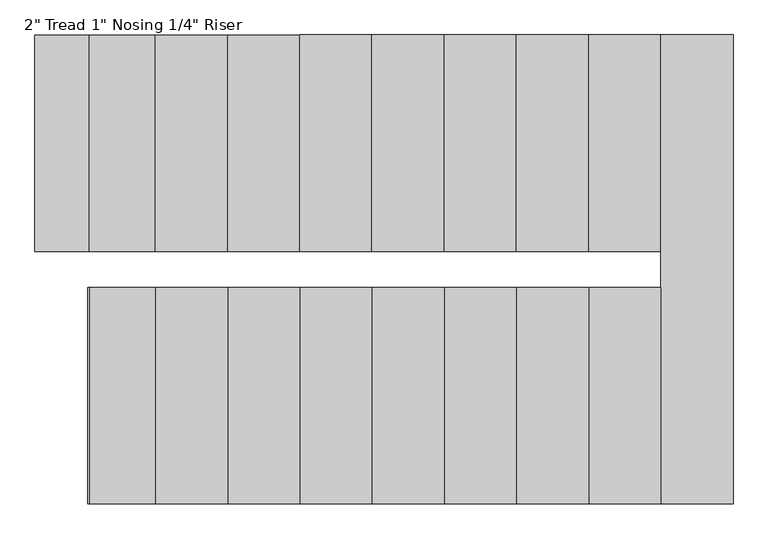
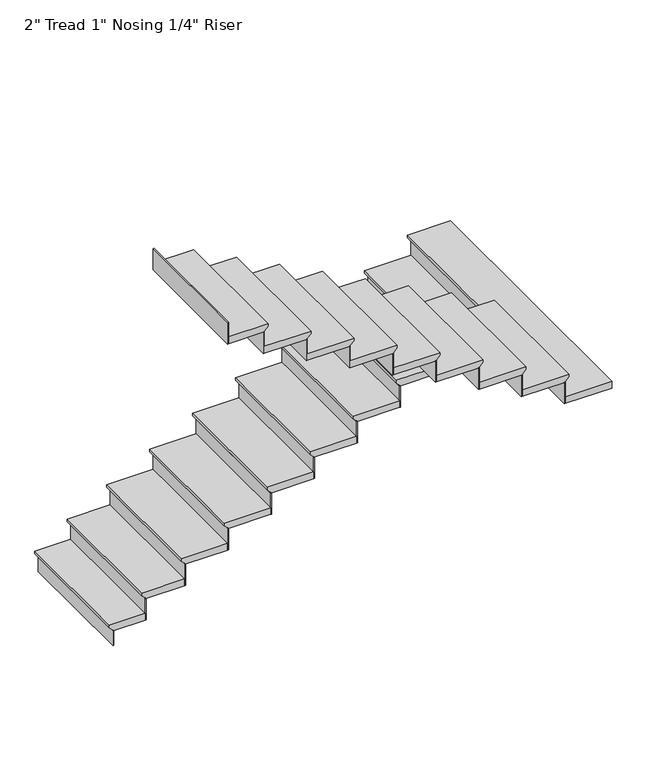
"""IFC4 building model written with IfcOpenShell, lengths in millimetres: stair flight geometry."""

from ifc_helpers import new_model, si_unit, origin, place, context, project, spatial, faceted_brep, source, transform, mapped, element, save


def stair_flight_a6cfe23b(model_context):
    return source(origin(), model_context, "Body", "Brep", [
        faceted_brep([(8572.5, 8280.4, 6237.3710526), (8572.5, 8280.4, 6256.4210526), (8572.5, 9194.8, 6256.4210526), (8572.5, 9194.8, 6237.3710526), (8597.9, 8280.4, 6211.9710526), (8597.9, 9194.8, 6211.9710526), (8826.5, 8280.4, 6256.4210526), (8826.5, 9194.8, 6256.4210526), (8597.9, 9194.8, 6205.6210526), (8826.5, 9194.8, 6205.6210526), (8826.5, 8280.4, 6205.6210526), (8597.9, 8280.4, 6205.6210526)], [[[0, 1, 2, 3]], [[4, 0, 3, 5]], [[2, 1, 6, 7]], [[8, 9, 10, 11]], [[2, 7, 9, 8, 5, 3]], [[8, 11, 4, 5]], [[6, 1, 0, 4, 11, 10]], [[7, 6, 10, 9]]]),
        faceted_brep([(8597.9, 8280.4, 6205.6210526), (8597.9, 8280.4, 6096.0), (8604.25, 8280.4, 6096.0), (8604.25, 8280.4, 6205.6210526), (8597.9, 9194.8, 6205.6210526), (8604.25, 9194.8, 6205.6210526), (8604.25, 9194.8, 6096.0), (8597.9, 9194.8, 6096.0)], [[[0, 1, 2, 3]], [[4, 5, 6, 7]], [[1, 0, 4, 7]], [[2, 1, 7, 6]], [[3, 2, 6, 5]], [[0, 3, 5, 4]]]),
        faceted_brep([(8826.5, 8280.4, 6366.0421053), (8826.5, 8280.4, 6205.6210526), (8832.85, 8280.4, 6205.6210526), (8832.85, 8280.4, 6366.0421053), (8826.5, 9194.8, 6366.0421053), (8832.85, 9194.8, 6366.0421053), (8832.85, 9194.8, 6205.6210526), (8826.5, 9194.8, 6205.6210526)], [[[0, 1, 2, 3]], [[4, 5, 6, 7]], [[1, 0, 4, 7]], [[2, 1, 7, 6]], [[3, 2, 6, 5]], [[0, 3, 5, 4]]]),
        faceted_brep([(8801.1, 9194.8, 6416.8421053), (8801.1, 8280.4, 6416.8421053), (9105.9, 8280.4, 6416.8421053), (9105.9, 9194.8, 6416.8421053), (8826.5, 9194.8, 6366.0421053), (9105.9, 9194.8, 6366.0421053), (9105.9, 8280.4, 6366.0421053), (8826.5, 8280.4, 6366.0421053), (8826.5, 9194.8, 6372.3921053), (8801.1, 9194.8, 6397.7921053), (8826.5, 8280.4, 6372.3921053), (8801.1, 8280.4, 6397.7921053)], [[[0, 1, 2, 3]], [[4, 5, 6, 7]], [[0, 3, 5, 4, 8, 9]], [[4, 7, 10, 8]], [[2, 1, 11, 10, 7, 6]], [[3, 2, 6, 5]], [[11, 1, 0, 9]], [[10, 11, 9, 8]]]),
        faceted_brep([(9105.9, 8280.4, 6526.4631579), (9105.9, 8280.4, 6366.0421053), (9112.25, 8280.4, 6366.0421053), (9112.25, 8280.4, 6526.4631579), (9105.9, 9194.8, 6526.4631579), (9112.25, 9194.8, 6526.4631579), (9112.25, 9194.8, 6366.0421053), (9105.9, 9194.8, 6366.0421053)], [[[0, 1, 2, 3]], [[4, 5, 6, 7]], [[1, 0, 4, 7]], [[2, 1, 7, 6]], [[3, 2, 6, 5]], [[0, 3, 5, 4]]]),
        faceted_brep([(9080.5, 9194.8, 6577.2631579), (9080.5, 8280.4, 6577.2631579), (9410.7, 8280.4, 6577.2631579), (9410.7, 9194.8, 6577.2631579), (9105.9, 9194.8, 6526.4631579), (9410.7, 9194.8, 6526.4631579), (9410.7, 8280.4, 6526.4631579), (9105.9, 8280.4, 6526.4631579), (9105.9, 9194.8, 6532.8131579), (9080.5, 9194.8, 6558.2131579), (9105.9, 8280.4, 6532.8131579), (9080.5, 8280.4, 6558.2131579)], [[[0, 1, 2, 3]], [[4, 5, 6, 7]], [[0, 3, 5, 4, 8, 9]], [[4, 7, 10, 8]], [[2, 1, 11, 10, 7, 6]], [[3, 2, 6, 5]], [[11, 1, 0, 9]], [[10, 11, 9, 8]]]),
        faceted_brep([(9410.7, 8280.4, 6686.8842105), (9410.7, 8280.4, 6526.4631579), (9417.05, 8280.4, 6526.4631579), (9417.05, 8280.4, 6686.8842105), (9410.7, 9194.8, 6686.8842105), (9417.05, 9194.8, 6686.8842105), (9417.05, 9194.8, 6526.4631579), (9410.7, 9194.8, 6526.4631579)], [[[0, 1, 2, 3]], [[4, 5, 6, 7]], [[1, 0, 4, 7]], [[2, 1, 7, 6]], [[3, 2, 6, 5]], [[0, 3, 5, 4]]]),
        faceted_brep([(9385.3, 9194.8, 6737.6842105), (9385.3, 8280.4, 6737.6842105), (9715.5, 8280.4, 6737.6842105), (9715.5, 9194.8, 6737.6842105), (9410.7, 9194.8, 6686.8842105), (9715.5, 9194.8, 6686.8842105), (9715.5, 8280.4, 6686.8842105), (9410.7, 8280.4, 6686.8842105), (9410.7, 9194.8, 6693.2342105), (9385.3, 9194.8, 6718.6342105), (9410.7, 8280.4, 6693.2342105), (9385.3, 8280.4, 6718.6342105)], [[[0, 1, 2, 3]], [[4, 5, 6, 7]], [[0, 3, 5, 4, 8, 9]], [[4, 7, 10, 8]], [[2, 1, 11, 10, 7, 6]], [[3, 2, 6, 5]], [[11, 1, 0, 9]], [[10, 11, 9, 8]]]),
        faceted_brep([(9715.5, 8280.4, 6847.3052632), (9715.5, 8280.4, 6686.8842105), (9721.85, 8280.4, 6686.8842105), (9721.85, 8280.4, 6847.3052632), (9715.5, 9194.8, 6847.3052632), (9721.85, 9194.8, 6847.3052632), (9721.85, 9194.8, 6686.8842105), (9715.5, 9194.8, 6686.8842105)], [[[0, 1, 2, 3]], [[4, 5, 6, 7]], [[1, 0, 4, 7]], [[2, 1, 7, 6]], [[3, 2, 6, 5]], [[0, 3, 5, 4]]]),
        faceted_brep([(9690.1, 9194.8, 6898.1052632), (9690.1, 8280.4, 6898.1052632), (10020.3, 8280.4, 6898.1052632), (10020.3, 9194.8, 6898.1052632), (9715.5, 9194.8, 6847.3052632), (10020.3, 9194.8, 6847.3052632), (10020.3, 8280.4, 6847.3052632), (9715.5, 8280.4, 6847.3052632), (9715.5, 9194.8, 6853.6552632), (9690.1, 9194.8, 6879.0552632), (9715.5, 8280.4, 6853.6552632), (9690.1, 8280.4, 6879.0552632)], [[[0, 1, 2, 3]], [[4, 5, 6, 7]], [[0, 3, 5, 4, 8, 9]], [[4, 7, 10, 8]], [[2, 1, 11, 10, 7, 6]], [[3, 2, 6, 5]], [[11, 1, 0, 9]], [[10, 11, 9, 8]]]),
        faceted_brep([(10020.3, 8280.4, 7007.7263158), (10020.3, 8280.4, 6847.3052632), (10026.65, 8280.4, 6847.3052632), (10026.65, 8280.4, 7007.7263158), (10020.3, 9194.8, 7007.7263158), (10026.65, 9194.8, 7007.7263158), (10026.65, 9194.8, 6847.3052632), (10020.3, 9194.8, 6847.3052632)], [[[0, 1, 2, 3]], [[4, 5, 6, 7]], [[1, 0, 4, 7]], [[2, 1, 7, 6]], [[3, 2, 6, 5]], [[0, 3, 5, 4]]]),
        faceted_brep([(9994.9, 9194.8, 7058.5263158), (9994.9, 8280.4, 7058.5263158), (10325.1, 8280.4, 7058.5263158), (10325.1, 9194.8, 7058.5263158), (10020.3, 9194.8, 7007.7263158), (10325.1, 9194.8, 7007.7263158), (10325.1, 8280.4, 7007.7263158), (10020.3, 8280.4, 7007.7263158), (10020.3, 9194.8, 7014.0763158), (9994.9, 9194.8, 7039.4763158), (10020.3, 8280.4, 7014.0763158), (9994.9, 8280.4, 7039.4763158)], [[[0, 1, 2, 3]], [[4, 5, 6, 7]], [[0, 3, 5, 4, 8, 9]], [[4, 7, 10, 8]], [[2, 1, 11, 10, 7, 6]], [[3, 2, 6, 5]], [[11, 1, 0, 9]], [[10, 11, 9, 8]]]),
        faceted_brep([(10325.1, 8280.4, 7168.1473684), (10325.1, 8280.4, 7007.7263158), (10331.45, 8280.4, 7007.7263158), (10331.45, 8280.4, 7168.1473684), (10325.1, 9194.8, 7168.1473684), (10331.45, 9194.8, 7168.1473684), (10331.45, 9194.8, 7007.7263158), (10325.1, 9194.8, 7007.7263158)], [[[0, 1, 2, 3]], [[4, 5, 6, 7]], [[1, 0, 4, 7]], [[2, 1, 7, 6]], [[3, 2, 6, 5]], [[0, 3, 5, 4]]]),
        faceted_brep([(10299.7, 9194.8, 7218.9473684), (10299.7, 8280.4, 7218.9473684), (10629.9, 8280.4, 7218.9473684), (10629.9, 9194.8, 7218.9473684), (10325.1, 9194.8, 7168.1473684), (10629.9, 9194.8, 7168.1473684), (10629.9, 8280.4, 7168.1473684), (10325.1, 8280.4, 7168.1473684), (10325.1, 9194.8, 7174.4973684), (10299.7, 9194.8, 7199.8973684), (10325.1, 8280.4, 7174.4973684), (10299.7, 8280.4, 7199.8973684)], [[[0, 1, 2, 3]], [[4, 5, 6, 7]], [[0, 3, 5, 4, 8, 9]], [[4, 7, 10, 8]], [[2, 1, 11, 10, 7, 6]], [[3, 2, 6, 5]], [[11, 1, 0, 9]], [[10, 11, 9, 8]]]),
        faceted_brep([(10629.9, 8280.4, 7328.5684211), (10629.9, 8280.4, 7168.1473684), (10636.25, 8280.4, 7168.1473684), (10636.25, 8280.4, 7328.5684211), (10629.9, 9194.8, 7328.5684211), (10636.25, 9194.8, 7328.5684211), (10636.25, 9194.8, 7168.1473684), (10629.9, 9194.8, 7168.1473684)], [[[0, 1, 2, 3]], [[4, 5, 6, 7]], [[1, 0, 4, 7]], [[2, 1, 7, 6]], [[3, 2, 6, 5]], [[0, 3, 5, 4]]]),
        faceted_brep([(10604.5, 9194.8, 7379.3684211), (10604.5, 8280.4, 7379.3684211), (10934.7, 8280.4, 7379.3684211), (10934.7, 9194.8, 7379.3684211), (10629.9, 9194.8, 7328.5684211), (10934.7, 9194.8, 7328.5684211), (10934.7, 8280.4, 7328.5684211), (10629.9, 8280.4, 7328.5684211), (10629.9, 9194.8, 7334.9184211), (10604.5, 9194.8, 7360.3184211), (10629.9, 8280.4, 7334.9184211), (10604.5, 8280.4, 7360.3184211)], [[[0, 1, 2, 3]], [[4, 5, 6, 7]], [[0, 3, 5, 4, 8, 9]], [[4, 7, 10, 8]], [[2, 1, 11, 10, 7, 6]], [[3, 2, 6, 5]], [[11, 1, 0, 9]], [[10, 11, 9, 8]]]),
        faceted_brep([(10934.7, 8280.4, 7488.9894737), (10934.7, 8280.4, 7328.5684211), (10941.05, 8280.4, 7328.5684211), (10941.05, 8280.4, 7488.9894737), (10934.7, 9194.8, 7488.9894737), (10941.05, 9194.8, 7488.9894737), (10941.05, 9194.8, 7328.5684211), (10934.7, 9194.8, 7328.5684211)], [[[0, 1, 2, 3]], [[4, 5, 6, 7]], [[1, 0, 4, 7]], [[2, 1, 7, 6]], [[3, 2, 6, 5]], [[0, 3, 5, 4]]]),
        faceted_brep([(10909.3, 9194.8, 7539.7894737), (10909.3, 8280.4, 7539.7894737), (11239.5, 8280.4, 7539.7894737), (11239.5, 9194.8, 7539.7894737), (10934.7, 9194.8, 7488.9894737), (11239.5, 9194.8, 7488.9894737), (11239.5, 8280.4, 7488.9894737), (10934.7, 8280.4, 7488.9894737), (10934.7, 9194.8, 7495.3394737), (10909.3, 9194.8, 7520.7394737), (10934.7, 8280.4, 7495.3394737), (10909.3, 8280.4, 7520.7394737)], [[[0, 1, 2, 3]], [[4, 5, 6, 7]], [[0, 3, 5, 4, 8, 9]], [[4, 7, 10, 8]], [[2, 1, 11, 10, 7, 6]], [[3, 2, 6, 5]], [[11, 1, 0, 9]], [[10, 11, 9, 8]]]),
        faceted_brep([(11239.5, 8280.4, 7649.4105263), (11239.5, 8280.4, 7488.9894737), (11245.85, 8280.4, 7488.9894737), (11245.85, 8280.4, 7649.4105263), (11239.5, 9194.8, 7649.4105263), (11245.85, 9194.8, 7649.4105263), (11245.85, 9194.8, 7488.9894737), (11239.5, 9194.8, 7488.9894737)], [[[0, 1, 2, 3]], [[4, 5, 6, 7]], [[1, 0, 4, 7]], [[2, 1, 7, 6]], [[3, 2, 6, 5]], [[0, 3, 5, 4]]]),
        faceted_brep([(11188.7, 7213.6, 7700.2105263), (11518.9, 7213.6, 7700.2105263), (11518.9, 9194.8, 7700.2105263), (11214.1, 9194.8, 7700.2105263), (11214.1, 8128.0, 7700.2105263), (11188.7, 8128.0, 7700.2105263), (11518.9, 7213.6, 7649.4105263), (11188.7, 7213.6, 7649.4105263), (11188.7, 8128.0, 7649.4105263), (11214.1, 8128.0, 7649.4105263), (11214.1, 8280.4, 7649.4105263), (11239.5, 8280.4, 7649.4105263), (11239.5, 9194.8, 7649.4105263), (11518.9, 9194.8, 7649.4105263), (11239.5, 9194.8, 7655.7605263), (11214.1, 9194.8, 7681.1605263), (11239.5, 8280.4, 7655.7605263), (11214.1, 8280.4, 7681.1605263)], [[[0, 1, 2, 3, 4, 5]], [[6, 7, 8, 9, 10, 11, 12, 13]], [[1, 0, 7, 6]], [[2, 1, 6, 13]], [[3, 2, 13, 12, 14, 15]], [[12, 11, 16, 14]], [[11, 10, 17, 16]], [[4, 3, 15, 17, 10, 9]], [[5, 4, 9, 8]], [[0, 5, 8, 7]], [[15, 14, 16, 17]]]),
        faceted_brep([(11188.7, 8128.0, 7809.8315789), (11188.7, 8128.0, 7649.4105263), (11182.35, 8128.0, 7649.4105263), (11182.35, 8128.0, 7809.8315789), (11188.7, 7213.6, 7809.8315789), (11182.35, 7213.6, 7809.8315789), (11182.35, 7213.6, 7649.4105263), (11188.7, 7213.6, 7649.4105263)], [[[0, 1, 2, 3]], [[4, 5, 6, 7]], [[1, 0, 4, 7]], [[2, 1, 7, 6]], [[3, 2, 6, 5]], [[0, 3, 5, 4]]]),
        faceted_brep([(11214.1, 7213.6, 7860.6315789), (11214.1, 8128.0, 7860.6315789), (10883.9, 8128.0, 7860.6315789), (10883.9, 7213.6, 7860.6315789), (11188.7, 7213.6, 7809.8315789), (10883.9, 7213.6, 7809.8315789), (10883.9, 8128.0, 7809.8315789), (11188.7, 8128.0, 7809.8315789), (11188.7, 7213.6, 7816.1815789), (11214.1, 7213.6, 7841.5815789), (11188.7, 8128.0, 7816.1815789), (11214.1, 8128.0, 7841.5815789)], [[[0, 1, 2, 3]], [[4, 5, 6, 7]], [[0, 3, 5, 4, 8, 9]], [[4, 7, 10, 8]], [[2, 1, 11, 10, 7, 6]], [[3, 2, 6, 5]], [[11, 1, 0, 9]], [[10, 11, 9, 8]]]),
        faceted_brep([(10883.9, 8128.0, 7970.2526316), (10883.9, 8128.0, 7809.8315789), (10877.55, 8128.0, 7809.8315789), (10877.55, 8128.0, 7970.2526316), (10883.9, 7213.6, 7970.2526316), (10877.55, 7213.6, 7970.2526316), (10877.55, 7213.6, 7809.8315789), (10883.9, 7213.6, 7809.8315789)], [[[0, 1, 2, 3]], [[4, 5, 6, 7]], [[1, 0, 4, 7]], [[2, 1, 7, 6]], [[3, 2, 6, 5]], [[0, 3, 5, 4]]]),
        faceted_brep([(10909.3, 7213.6, 8021.0526316), (10909.3, 8128.0, 8021.0526316), (10579.1, 8128.0, 8021.0526316), (10579.1, 7213.6, 8021.0526316), (10883.9, 7213.6, 7970.2526316), (10579.1, 7213.6, 7970.2526316), (10579.1, 8128.0, 7970.2526316), (10883.9, 8128.0, 7970.2526316), (10883.9, 7213.6, 7976.6026316), (10909.3, 7213.6, 8002.0026316), (10883.9, 8128.0, 7976.6026316), (10909.3, 8128.0, 8002.0026316)], [[[0, 1, 2, 3]], [[4, 5, 6, 7]], [[0, 3, 5, 4, 8, 9]], [[4, 7, 10, 8]], [[2, 1, 11, 10, 7, 6]], [[3, 2, 6, 5]], [[11, 1, 0, 9]], [[10, 11, 9, 8]]]),
        faceted_brep([(10579.1, 8128.0, 8130.6736842), (10579.1, 8128.0, 7970.2526316), (10572.75, 8128.0, 7970.2526316), (10572.75, 8128.0, 8130.6736842), (10579.1, 7213.6, 8130.6736842), (10572.75, 7213.6, 8130.6736842), (10572.75, 7213.6, 7970.2526316), (10579.1, 7213.6, 7970.2526316)], [[[0, 1, 2, 3]], [[4, 5, 6, 7]], [[1, 0, 4, 7]], [[2, 1, 7, 6]], [[3, 2, 6, 5]], [[0, 3, 5, 4]]]),
        faceted_brep([(10604.5, 7213.6, 8181.4736842), (10604.5, 8128.0, 8181.4736842), (10274.3, 8128.0, 8181.4736842), (10274.3, 7213.6, 8181.4736842), (10579.1, 7213.6, 8130.6736842), (10274.3, 7213.6, 8130.6736842), (10274.3, 8128.0, 8130.6736842), (10579.1, 8128.0, 8130.6736842), (10579.1, 7213.6, 8137.0236842), (10604.5, 7213.6, 8162.4236842), (10579.1, 8128.0, 8137.0236842), (10604.5, 8128.0, 8162.4236842)], [[[0, 1, 2, 3]], [[4, 5, 6, 7]], [[0, 3, 5, 4, 8, 9]], [[4, 7, 10, 8]], [[2, 1, 11, 10, 7, 6]], [[3, 2, 6, 5]], [[11, 1, 0, 9]], [[10, 11, 9, 8]]]),
        faceted_brep([(10274.3, 8128.0, 8291.0947368), (10274.3, 8128.0, 8130.6736842), (10267.95, 8128.0, 8130.6736842), (10267.95, 8128.0, 8291.0947368), (10274.3, 7213.6, 8291.0947368), (10267.95, 7213.6, 8291.0947368), (10267.95, 7213.6, 8130.6736842), (10274.3, 7213.6, 8130.6736842)], [[[0, 1, 2, 3]], [[4, 5, 6, 7]], [[1, 0, 4, 7]], [[2, 1, 7, 6]], [[3, 2, 6, 5]], [[0, 3, 5, 4]]]),
        faceted_brep([(10299.7, 7213.6, 8341.8947368), (10299.7, 8128.0, 8341.8947368), (9969.5, 8128.0, 8341.8947368), (9969.5, 7213.6, 8341.8947368), (10274.3, 7213.6, 8291.0947368), (9969.5, 7213.6, 8291.0947368), (9969.5, 8128.0, 8291.0947368), (10274.3, 8128.0, 8291.0947368), (10274.3, 7213.6, 8297.4447368), (10299.7, 7213.6, 8322.8447368), (10274.3, 8128.0, 8297.4447368), (10299.7, 8128.0, 8322.8447368)], [[[0, 1, 2, 3]], [[4, 5, 6, 7]], [[0, 3, 5, 4, 8, 9]], [[4, 7, 10, 8]], [[2, 1, 11, 10, 7, 6]], [[3, 2, 6, 5]], [[11, 1, 0, 9]], [[10, 11, 9, 8]]]),
        faceted_brep([(9969.5, 8128.0, 8451.5157895), (9969.5, 8128.0, 8291.0947368), (9963.15, 8128.0, 8291.0947368), (9963.15, 8128.0, 8451.5157895), (9969.5, 7213.6, 8451.5157895), (9963.15, 7213.6, 8451.5157895), (9963.15, 7213.6, 8291.0947368), (9969.5, 7213.6, 8291.0947368)], [[[0, 1, 2, 3]], [[4, 5, 6, 7]], [[1, 0, 4, 7]], [[2, 1, 7, 6]], [[3, 2, 6, 5]], [[0, 3, 5, 4]]]),
        faceted_brep([(9994.9, 7213.6, 8502.3157895), (9994.9, 8128.0, 8502.3157895), (9664.7, 8128.0, 8502.3157895), (9664.7, 7213.6, 8502.3157895), (9969.5, 7213.6, 8451.5157895), (9664.7, 7213.6, 8451.5157895), (9664.7, 8128.0, 8451.5157895), (9969.5, 8128.0, 8451.5157895), (9969.5, 7213.6, 8457.8657895), (9994.9, 7213.6, 8483.2657895), (9969.5, 8128.0, 8457.8657895), (9994.9, 8128.0, 8483.2657895)], [[[0, 1, 2, 3]], [[4, 5, 6, 7]], [[0, 3, 5, 4, 8, 9]], [[4, 7, 10, 8]], [[2, 1, 11, 10, 7, 6]], [[3, 2, 6, 5]], [[11, 1, 0, 9]], [[10, 11, 9, 8]]]),
        faceted_brep([(9664.7, 8128.0, 8611.9368421), (9664.7, 8128.0, 8451.5157895), (9658.35, 8128.0, 8451.5157895), (9658.35, 8128.0, 8611.9368421), (9664.7, 7213.6, 8611.9368421), (9658.35, 7213.6, 8611.9368421), (9658.35, 7213.6, 8451.5157895), (9664.7, 7213.6, 8451.5157895)], [[[0, 1, 2, 3]], [[4, 5, 6, 7]], [[1, 0, 4, 7]], [[2, 1, 7, 6]], [[3, 2, 6, 5]], [[0, 3, 5, 4]]]),
        faceted_brep([(9690.1, 7213.6, 8662.7368421), (9690.1, 8128.0, 8662.7368421), (9359.9, 8128.0, 8662.7368421), (9359.9, 7213.6, 8662.7368421), (9664.7, 7213.6, 8611.9368421), (9359.9, 7213.6, 8611.9368421), (9359.9, 8128.0, 8611.9368421), (9664.7, 8128.0, 8611.9368421), (9664.7, 7213.6, 8618.2868421), (9690.1, 7213.6, 8643.6868421), (9664.7, 8128.0, 8618.2868421), (9690.1, 8128.0, 8643.6868421)], [[[0, 1, 2, 3]], [[4, 5, 6, 7]], [[0, 3, 5, 4, 8, 9]], [[4, 7, 10, 8]], [[2, 1, 11, 10, 7, 6]], [[3, 2, 6, 5]], [[11, 1, 0, 9]], [[10, 11, 9, 8]]]),
        faceted_brep([(9359.9, 8128.0, 8772.3578947), (9359.9, 8128.0, 8611.9368421), (9353.55, 8128.0, 8611.9368421), (9353.55, 8128.0, 8772.3578947), (9359.9, 7213.6, 8772.3578947), (9353.55, 7213.6, 8772.3578947), (9353.55, 7213.6, 8611.9368421), (9359.9, 7213.6, 8611.9368421)], [[[0, 1, 2, 3]], [[4, 5, 6, 7]], [[1, 0, 4, 7]], [[2, 1, 7, 6]], [[3, 2, 6, 5]], [[0, 3, 5, 4]]]),
        faceted_brep([(9385.3, 7213.6, 8823.1578947), (9385.3, 8128.0, 8823.1578947), (9055.1, 8128.0, 8823.1578947), (9055.1, 7213.6, 8823.1578947), (9359.9, 7213.6, 8772.3578947), (9055.1, 7213.6, 8772.3578947), (9055.1, 8128.0, 8772.3578947), (9359.9, 8128.0, 8772.3578947), (9359.9, 7213.6, 8778.7078947), (9385.3, 7213.6, 8804.1078947), (9359.9, 8128.0, 8778.7078947), (9385.3, 8128.0, 8804.1078947)], [[[0, 1, 2, 3]], [[4, 5, 6, 7]], [[0, 3, 5, 4, 8, 9]], [[4, 7, 10, 8]], [[2, 1, 11, 10, 7, 6]], [[3, 2, 6, 5]], [[11, 1, 0, 9]], [[10, 11, 9, 8]]]),
        faceted_brep([(9055.1, 8128.0, 8932.7789474), (9055.1, 8128.0, 8772.3578947), (9048.75, 8128.0, 8772.3578947), (9048.75, 8128.0, 8932.7789474), (9055.1, 7213.6, 8932.7789474), (9048.75, 7213.6, 8932.7789474), (9048.75, 7213.6, 8772.3578947), (9055.1, 7213.6, 8772.3578947)], [[[0, 1, 2, 3]], [[4, 5, 6, 7]], [[1, 0, 4, 7]], [[2, 1, 7, 6]], [[3, 2, 6, 5]], [[0, 3, 5, 4]]]),
        faceted_brep([(8801.1, 8128.0, 9093.2), (8801.1, 8128.0, 8932.7789474), (8794.75, 8128.0, 8932.7789474), (8794.75, 8128.0, 9093.2), (8801.1, 7213.6, 9093.2), (8794.75, 7213.6, 9093.2), (8794.75, 7213.6, 8932.7789474), (8801.1, 7213.6, 8932.7789474)], [[[0, 1, 2, 3]], [[4, 5, 6, 7]], [[1, 0, 4, 7]], [[2, 1, 7, 6]], [[3, 2, 6, 5]], [[0, 3, 5, 4]]]),
        faceted_brep([(9080.5, 7213.6, 8983.5789474), (9080.5, 8128.0, 8983.5789474), (8801.1, 8128.0, 8983.5789474), (8801.1, 7213.6, 8983.5789474), (9055.1, 7213.6, 8932.7789474), (8801.1, 7213.6, 8932.7789474), (8801.1, 8128.0, 8932.7789474), (9055.1, 8128.0, 8932.7789474), (9055.1, 7213.6, 8939.1289474), (9080.5, 7213.6, 8964.5289474), (9055.1, 8128.0, 8939.1289474), (9080.5, 8128.0, 8964.5289474)], [[[0, 1, 2, 3]], [[4, 5, 6, 7]], [[0, 3, 5, 4, 8, 9]], [[4, 7, 10, 8]], [[2, 1, 11, 10, 7, 6]], [[3, 2, 6, 5]], [[11, 1, 0, 9]], [[10, 11, 9, 8]]]),
    ])


if __name__ == "__main__":
    model = new_model("IFC4")
    model_context = context("Model", 3, world=origin())
    ifc_project = project(units=[si_unit("LENGTHUNIT", "METRE", prefix="MILLI")], contexts=[model_context])
    site = spatial("IfcSite", under=ifc_project)
    building = spatial("IfcBuilding", under=site)
    placement = place(None, origin())
    stair_flight_shape = stair_flight_a6cfe23b(model_context)
    element("IfcStairFlight", 1, ObjectType="2\" Tread 1\" Nosing 1/4\" Riser", at=placement, inside=building, context=model_context, shape_type="MappedRepresentation", body=[
        mapped(stair_flight_shape, transform((0.0, 0.0, 0.0), x_axis=(1.0, 0.0, 0.0), y_axis=(0.0, 1.0, 0.0), z_axis=(0.0, 0.0, 1.0))),
    ])
    save(model, "model.ifc")
